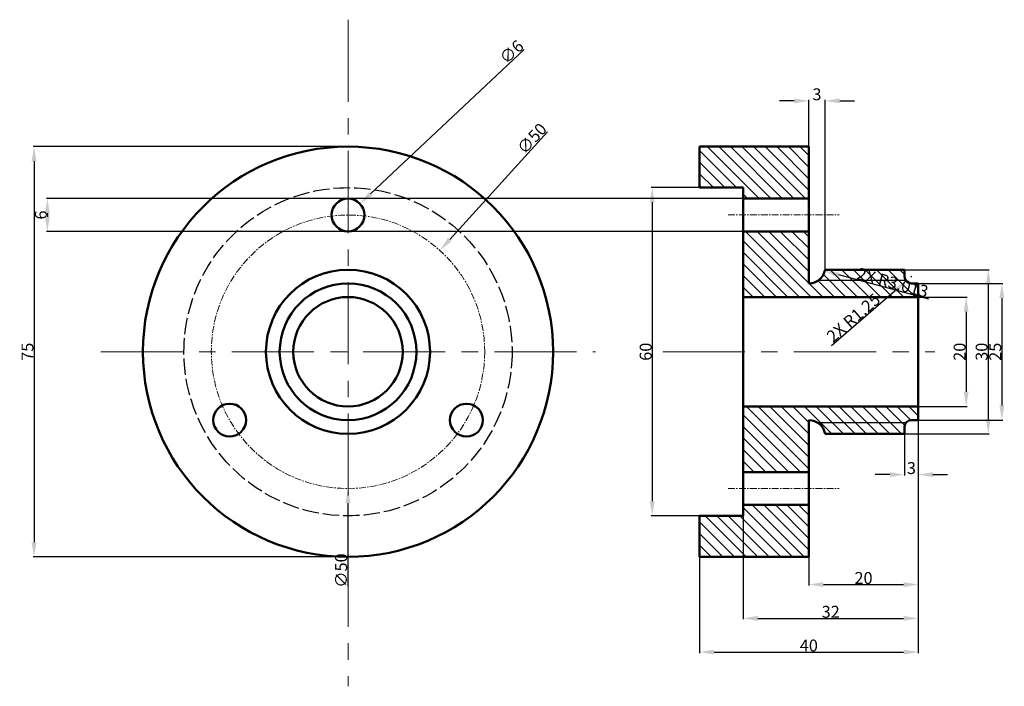
# Model space of a CAD drawing. Units: millimetres. Extents: x 379 to 559, y 190 to 312.
import ezdxf

# ---------------------------------------------------------------- set-up
doc = ezdxf.new("R2010")
doc.units = ezdxf.units.MM
doc.header["$MEASUREMENT"] = 0
doc.linetypes.add('ACAD_ISO02W100', pattern=[15, 12, -3])
doc.linetypes.add('CENTER', pattern=[2, 1.25, -0.25, 0.25, -0.25])
for name, color, linetype, lineweight in [('M-CNTR', 4, 'CENTER', 18), ('M-DIMS', 2, 'Continuous', 25), ('M-HATC', 8, 'Continuous', 18), ('M-HIDN', 3, 'ACAD_ISO02W100', 25), ('M-OUTL', 7, 'Continuous', 50), ('M-THRD', 7, 'Continuous', 25)]:
    doc.layers.add(name, color=color, linetype=linetype, lineweight=lineweight)
doc.styles.get("Standard").update_dxf_attribs({"font": 'arial.ttf'})
doc.dimstyles.get("Standard").update_dxf_attribs({"dimtxt": 2.18, "dimasz": 2.68, "dimexe": 0.18, "dimexo": 0.0625, "dimgap": 0.09, "dimtad": 1, "dimdec": 0, "dimzin": 0, "dimdsep": 46, "dimtxsty": 'Standard', "dimcen": 0.09, "dimadec": 0, "dimazin": 0, "dimtfac": 1, "dimtdec": 0, "dimtofl": 0, "dimtmove": 0, "dimatfit": 3, "dimfxl": 1, "dimtolj": 1, "dimtzin": 0, "dimarcsym": 0})

# ---------------------------------------------------------------- blocks, each defined once
blk = doc.blocks.new('*U1')
blk.add_circle((0, 0), 3)
blk = doc.blocks.new('*U2')
at = {"layer": 'M-OUTL', "color": 0, "linetype": 'ByBlock', "lineweight": -2, "transparency": 16777216}
blk.add_blockref('*U1', (438.8, 276.4), dxfattribs=at)
for p, rotation in [((417.15, 238.9), 120), ((460.45, 238.9), 240)]:
    blk.add_blockref('*U1', p, dxfattribs=dict(at, rotation=rotation))
blk = doc.blocks.new('*D3')
at = {"layer": 'Defpoints', "color": 0, "transparency": 16777216}
for p in [(438.8, 288.9), (381.39, 213.9), (438.8, 213.9)]:
    blk.add_point(p, dxfattribs=at)
at = {"layer": 'M-DIMS', "color": 0, "lineweight": -2, "transparency": 16777216}
for p, q in [((438.74, 288.9), (381.21, 288.9)), ((381.39, 286.22), (381.39, 216.58)), ((438.74, 213.9), (381.21, 213.9))]:
    blk.add_line(p, q, dxfattribs=at)
at = {"layer": 'M-DIMS', "color": 0, "transparency": 16777216}
for points in [[(380.94, 286.22), (381.84, 286.22), (381.39, 288.9)], [(380.94, 216.58), (381.84, 216.58), (381.39, 213.9)]]:
    blk.add_solid(points, dxfattribs=at)
at = {"layer": 'M-DIMS', "color": 0, "transparency": 16777216, "insert": (380.19, 251.4), "char_height": 2.18, "attachment_point": 5, "rotation": 90}
blk.add_mtext('\\A1;75', dxfattribs=at)
blk = doc.blocks.new('*D4')
at = {"layer": 'Defpoints', "color": 0, "transparency": 16777216}
for p in [(440.99, 278.45), (436.61, 274.34)]:
    blk.add_point(p, dxfattribs=at)
at = {"layer": 'M-DIMS', "color": 0, "lineweight": -2, "transparency": 16777216}
for p, q in [((471.01, 306.65), (442.94, 280.29)), ((438.71, 276.4), (438.89, 276.4)), ((438.8, 276.31), (438.8, 276.49))]:
    blk.add_line(p, q, dxfattribs=at)
at = {"layer": 'M-DIMS', "color": 0, "transparency": 16777216}
blk.add_solid([(442.64, 280.61), (443.25, 279.96), (440.99, 278.45)], dxfattribs=at)
at = {"layer": 'M-DIMS', "color": 0, "transparency": 16777216, "insert": (468.7, 306.21), "char_height": 2.18, "attachment_point": 5, "rotation": 43.2019}
blk.add_mtext('\\A1;∅6', dxfattribs=at)
blk = doc.blocks.new('*D5')
at = {"layer": 'Defpoints', "color": 0, "transparency": 16777216}
for p in [(503.07, 281.4), (494.44, 221.4), (503.07, 221.4)]:
    blk.add_point(p, dxfattribs=at)
at = {"layer": 'M-DIMS', "color": 0, "lineweight": -2, "transparency": 16777216}
for p, q in [((503, 281.4), (494.26, 281.4)), ((494.44, 278.72), (494.44, 224.08)), ((503, 221.4), (494.26, 221.4))]:
    blk.add_line(p, q, dxfattribs=at)
at = {"layer": 'M-DIMS', "color": 0, "transparency": 16777216}
for points in [[(493.99, 278.72), (494.88, 278.72), (494.44, 281.4)], [(493.99, 224.08), (494.88, 224.08), (494.44, 221.4)]]:
    blk.add_solid(points, dxfattribs=at)
at = {"layer": 'M-DIMS', "color": 0, "transparency": 16777216, "insert": (493.23, 251.4), "char_height": 2.18, "attachment_point": 5, "rotation": 90}
blk.add_mtext('\\A1;60', dxfattribs=at)
blk = doc.blocks.new('*D6')
at = {"layer": 'Defpoints', "color": 0, "transparency": 16777216}
for p in [(523.07, 297.26), (523.07, 266.4), (526.03, 266.4)]:
    blk.add_point(p, dxfattribs=at)
at = {"layer": 'M-DIMS', "color": 0, "lineweight": -2, "transparency": 16777216}
for p, q in [((520.39, 297.26), (517.71, 297.26)), ((523.07, 266.46), (523.07, 297.44)), ((526.03, 266.46), (526.03, 297.44)), ((528.71, 297.26), (531.39, 297.26))]:
    blk.add_line(p, q, dxfattribs=at)
at = {"layer": 'M-DIMS', "color": 0, "transparency": 16777216}
for points in [[(520.39, 297.71), (520.39, 296.81), (523.07, 297.26)], [(528.71, 297.71), (528.71, 296.81), (526.03, 297.26)]]:
    blk.add_solid(points, dxfattribs=at)
at = {"layer": 'M-DIMS', "color": 0, "transparency": 16777216, "insert": (524.55, 298.46), "char_height": 2.18, "attachment_point": 5}
blk.add_mtext('\\A1;3', dxfattribs=at)
blk = doc.blocks.new('*D7')
at = {"layer": 'Defpoints', "color": 0, "transparency": 16777216}
for p in [(543.07, 261.4), (543.07, 241.4), (551.84, 241.4)]:
    blk.add_point(p, dxfattribs=at)
at = {"layer": 'M-DIMS', "color": 0, "lineweight": -2, "transparency": 16777216}
for p, q in [((543.13, 261.4), (552.02, 261.4)), ((551.84, 258.72), (551.84, 244.08)), ((543.13, 241.4), (552.02, 241.4))]:
    blk.add_line(p, q, dxfattribs=at)
at = {"layer": 'M-DIMS', "color": 0, "transparency": 16777216}
for points in [[(551.39, 258.72), (552.29, 258.72), (551.84, 261.4)], [(551.39, 244.08), (552.29, 244.08), (551.84, 241.4)]]:
    blk.add_solid(points, dxfattribs=at)
at = {"layer": 'M-DIMS', "color": 0, "transparency": 16777216, "insert": (550.64, 251.4), "char_height": 2.18, "attachment_point": 5, "rotation": 90}
blk.add_mtext('\\A1;20', dxfattribs=at)
blk = doc.blocks.new('*D8')
at = {"layer": 'Defpoints', "color": 0, "transparency": 16777216}
for p in [(543.07, 263.9), (543.07, 238.9), (558.37, 238.9)]:
    blk.add_point(p, dxfattribs=at)
at = {"layer": 'M-DIMS', "color": 0, "lineweight": -2, "transparency": 16777216}
for p, q in [((543.13, 263.9), (558.55, 263.9)), ((558.37, 261.22), (558.37, 241.58)), ((543.13, 238.9), (558.55, 238.9))]:
    blk.add_line(p, q, dxfattribs=at)
at = {"layer": 'M-DIMS', "color": 0, "transparency": 16777216}
for points in [[(557.92, 261.22), (558.81, 261.22), (558.37, 263.9)], [(557.92, 241.58), (558.81, 241.58), (558.37, 238.9)]]:
    blk.add_solid(points, dxfattribs=at)
at = {"layer": 'M-DIMS', "color": 0, "transparency": 16777216, "insert": (557.16, 251.4), "char_height": 2.18, "attachment_point": 5, "rotation": 90}
blk.add_mtext('\\A1;25', dxfattribs=at)
blk = doc.blocks.new('*D9')
at = {"layer": 'Defpoints', "color": 0, "transparency": 16777216}
for p in [(543.07, 238.9), (540.57, 236.4), (543.07, 228.93)]:
    blk.add_point(p, dxfattribs=at)
at = {"layer": 'M-DIMS', "color": 0, "lineweight": -2, "transparency": 16777216}
for p, q in [((543.07, 238.84), (543.07, 228.75)), ((540.57, 236.34), (540.57, 228.75)), ((537.89, 228.93), (535.21, 228.93)), ((545.75, 228.93), (548.43, 228.93))]:
    blk.add_line(p, q, dxfattribs=at)
at = {"layer": 'M-DIMS', "color": 0, "transparency": 16777216}
for points in [[(537.89, 229.38), (537.89, 228.48), (540.57, 228.93)], [(545.75, 229.38), (545.75, 228.48), (543.07, 228.93)]]:
    blk.add_solid(points, dxfattribs=at)
at = {"layer": 'M-DIMS', "color": 0, "transparency": 16777216, "insert": (541.82, 230.13), "char_height": 2.18, "attachment_point": 5}
blk.add_mtext('\\A1;3', dxfattribs=at)
blk = doc.blocks.new('*D10')
at = {"layer": 'Defpoints', "color": 0, "transparency": 16777216}
for p in [(543.07, 238.9), (523.07, 213.9), (543.07, 208.84)]:
    blk.add_point(p, dxfattribs=at)
at = {"layer": 'M-DIMS', "color": 0, "lineweight": -2, "transparency": 16777216}
for p, q in [((543.07, 238.84), (543.07, 208.66)), ((523.07, 213.84), (523.07, 208.66)), ((525.75, 208.84), (540.39, 208.84))]:
    blk.add_line(p, q, dxfattribs=at)
at = {"layer": 'M-DIMS', "color": 0, "transparency": 16777216}
for points in [[(525.75, 209.28), (525.75, 208.39), (523.07, 208.84)], [(540.39, 209.28), (540.39, 208.39), (543.07, 208.84)]]:
    blk.add_solid(points, dxfattribs=at)
at = {"layer": 'M-DIMS', "color": 0, "transparency": 16777216, "insert": (533.07, 210.04), "char_height": 2.18, "attachment_point": 5}
blk.add_mtext('\\A1;20', dxfattribs=at)
blk = doc.blocks.new('*D11')
at = {"layer": 'Defpoints', "color": 0, "transparency": 16777216}
for p in [(543.07, 238.9), (511.07, 221.4), (543.07, 202.66)]:
    blk.add_point(p, dxfattribs=at)
at = {"layer": 'M-DIMS', "color": 0, "lineweight": -2, "transparency": 16777216}
for p, q in [((543.07, 238.84), (543.07, 202.48)), ((511.07, 221.34), (511.07, 202.48)), ((513.75, 202.66), (540.39, 202.66))]:
    blk.add_line(p, q, dxfattribs=at)
at = {"layer": 'M-DIMS', "color": 0, "transparency": 16777216}
for points in [[(513.75, 203.1), (513.75, 202.21), (511.07, 202.66)], [(540.39, 203.1), (540.39, 202.21), (543.07, 202.66)]]:
    blk.add_solid(points, dxfattribs=at)
at = {"layer": 'M-DIMS', "color": 0, "transparency": 16777216, "insert": (527.07, 203.86), "char_height": 2.18, "attachment_point": 5}
blk.add_mtext('\\A1;32', dxfattribs=at)
blk = doc.blocks.new('*D12')
at = {"layer": 'Defpoints', "color": 0, "transparency": 16777216}
for p in [(543.07, 238.9), (503.07, 213.9), (543.07, 196.5)]:
    blk.add_point(p, dxfattribs=at)
at = {"layer": 'M-DIMS', "color": 0, "lineweight": -2, "transparency": 16777216}
for p, q in [((543.07, 238.84), (543.07, 196.32)), ((503.07, 213.84), (503.07, 196.32)), ((505.75, 196.5), (540.39, 196.5))]:
    blk.add_line(p, q, dxfattribs=at)
at = {"layer": 'M-DIMS', "color": 0, "transparency": 16777216}
for points in [[(505.75, 196.95), (505.75, 196.05), (503.07, 196.5)], [(540.39, 196.95), (540.39, 196.05), (543.07, 196.5)]]:
    blk.add_solid(points, dxfattribs=at)
at = {"layer": 'M-DIMS', "color": 0, "transparency": 16777216, "insert": (523.07, 197.7), "char_height": 2.18, "attachment_point": 5}
blk.add_mtext('\\A1;40', dxfattribs=at)
blk = doc.blocks.new('*D13')
at = {"layer": 'Defpoints', "color": 0, "transparency": 16777216}
for p in [(455.6, 269.92), (422.01, 232.88)]:
    blk.add_point(p, dxfattribs=at)
at = {"layer": 'M-DIMS', "color": 0, "lineweight": -2, "transparency": 16777216}
for p, q in [((475.27, 291.62), (457.4, 271.9)), ((438.71, 251.4), (438.89, 251.4)), ((438.8, 251.31), (438.8, 251.49))]:
    blk.add_line(p, q, dxfattribs=at)
at = {"layer": 'M-DIMS', "color": 0, "transparency": 16777216}
blk.add_solid([(457.07, 272.2), (457.73, 271.6), (455.6, 269.92)], dxfattribs=at)
at = {"layer": 'M-DIMS', "color": 0, "transparency": 16777216, "insert": (472.43, 290.37), "char_height": 2.18, "attachment_point": 5, "rotation": 47.7955}
blk.add_mtext('\\A1;∅50', dxfattribs=at)
blk = doc.blocks.new('*D14')
at = {"layer": 'Defpoints', "color": 0, "transparency": 16777216}
for p in [(511.07, 279.4), (383.82, 273.4), (511.07, 273.4)]:
    blk.add_point(p, dxfattribs=at)
at = {"layer": 'M-DIMS', "color": 0, "lineweight": -2, "transparency": 16777216}
for p, q in [((511, 279.4), (383.64, 279.4)), ((383.82, 276.72), (383.82, 276.08)), ((511, 273.4), (383.64, 273.4))]:
    blk.add_line(p, q, dxfattribs=at)
at = {"layer": 'M-DIMS', "color": 0, "transparency": 16777216}
for points in [[(383.37, 276.72), (384.27, 276.72), (383.82, 279.4)], [(383.37, 276.08), (384.27, 276.08), (383.82, 273.4)]]:
    blk.add_solid(points, dxfattribs=at)
at = {"layer": 'M-DIMS', "color": 0, "transparency": 16777216, "insert": (382.62, 276.4), "char_height": 2.18, "attachment_point": 5, "rotation": 90}
blk.add_mtext('\\A1;6', dxfattribs=at)
blk = doc.blocks.new('*D15')
at = {"layer": 'Defpoints', "color": 0, "transparency": 16777216}
for p in [(540.57, 266.4), (540.57, 236.4), (555.88, 236.4)]:
    blk.add_point(p, dxfattribs=at)
at = {"layer": 'M-DIMS', "color": 0, "lineweight": -2, "transparency": 16777216}
for p, q in [((540.63, 266.4), (556.06, 266.4)), ((555.88, 263.72), (555.88, 239.08)), ((540.63, 236.4), (556.06, 236.4))]:
    blk.add_line(p, q, dxfattribs=at)
at = {"layer": 'M-DIMS', "color": 0, "transparency": 16777216}
for points in [[(555.43, 263.72), (556.33, 263.72), (555.88, 266.4)], [(555.43, 239.08), (556.33, 239.08), (555.88, 236.4)]]:
    blk.add_solid(points, dxfattribs=at)
at = {"layer": 'M-DIMS', "color": 0, "transparency": 16777216, "insert": (554.67, 251.4), "char_height": 2.18, "attachment_point": 5, "rotation": 90}
blk.add_mtext('\\A1;30', dxfattribs=at)
blk = doc.blocks.new('*D16')
at = {"layer": 'Defpoints', "color": 0, "transparency": 16777216}
for p in [(438.8, 276.4), (438.8, 226.4)]:
    blk.add_point(p, dxfattribs=at)
at = {"layer": 'M-DIMS', "color": 0, "lineweight": -2, "transparency": 16777216}
for p, q in [((438.71, 251.4), (438.89, 251.4)), ((438.8, 251.31), (438.8, 251.49)), ((438.8, 208.56), (438.8, 223.72))]:
    blk.add_line(p, q, dxfattribs=at)
at = {"layer": 'M-DIMS', "color": 0, "transparency": 16777216}
blk.add_solid([(438.35, 223.72), (439.25, 223.72), (438.8, 226.4)], dxfattribs=at)
at = {"layer": 'M-DIMS', "color": 0, "transparency": 16777216, "insert": (437.54, 211.4), "char_height": 2.18, "attachment_point": 5, "rotation": 89.997}
blk.add_mtext('\\A1;∅50', dxfattribs=at)
blk = doc.blocks.new('*D17')
at = {"layer": 'Defpoints', "color": 0, "transparency": 16777216}
for p in [(523.07, 266.91), (525.97, 266.13)]:
    blk.add_point(p, dxfattribs=at)
at = {"layer": 'M-DIMS', "color": 0, "lineweight": -2, "transparency": 16777216}
for p, q in [((522.98, 266.91), (523.16, 266.91)), ((523.07, 266.82), (523.07, 267)), ((545, 261.01), (528.56, 265.43))]:
    blk.add_line(p, q, dxfattribs=at)
at = {"layer": 'M-DIMS', "color": 0, "transparency": 16777216}
blk.add_solid([(528.68, 265.86), (528.45, 265), (525.97, 266.13)], dxfattribs=at)
at = {"layer": 'M-DIMS', "color": 0, "transparency": 16777216, "insert": (538.39, 264.04), "char_height": 2.18, "attachment_point": 5, "rotation": 344.9428}
blk.add_mtext('\\A1;2X R3.013', dxfattribs=at)
blk = doc.blocks.new('*D18')
at = {"layer": 'Defpoints', "color": 0, "transparency": 16777216}
for p in [(541.82, 265.15), (540.87, 264.33)]:
    blk.add_point(p, dxfattribs=at)
at = {"layer": 'M-DIMS', "color": 0, "lineweight": -2, "transparency": 16777216}
for p, q in [((541.73, 265.15), (541.91, 265.15)), ((541.82, 265.06), (541.82, 265.24)), ((527.21, 252.57), (538.84, 262.58))]:
    blk.add_line(p, q, dxfattribs=at)
at = {"layer": 'M-DIMS', "color": 0, "transparency": 16777216}
blk.add_solid([(538.55, 262.92), (539.13, 262.24), (540.87, 264.33)], dxfattribs=at)
at = {"layer": 'M-DIMS', "color": 0, "transparency": 16777216, "insert": (531.22, 257.61), "char_height": 2.18, "attachment_point": 5, "rotation": 40.7501}
blk.add_mtext('\\A1;2X R1.25', dxfattribs=at)

msp = doc.modelspace()

# ---------------------------------------------------------------- hatches: boundary and pattern name
at = {"layer": 'M-HATC'}
h = msp.add_hatch(dxfattribs=at)
h.set_pattern_fill('ANSI31', color=256, scale=12, angle=90)
h.paths.add_polyline_path([(523.0651, 288.8985), (503.0651, 288.8985), (503.0651, 281.3985), (511.0651, 281.3985), (511.0651, 279.3985), (523.0651, 279.3985)])
h = msp.add_hatch(dxfattribs=at)
h.set_pattern_fill('ANSI31', color=256, scale=12, angle=90)
h.paths.add_polyline_path([(523.0651, 273.3985), (511.0651, 273.3985), (511.0651, 261.3985), (543.0651, 261.3985), (543.0651, 263.8985), (541.8151, 263.8985, -0.23606798), (540.8151, 264.3985), (524.7273, 264.3985, -0.14714445), (523.0651, 263.8985)])
h.paths.add_polyline_path([(523.0651, 238.8985, -0.14714445), (524.7273, 238.3985), (540.8151, 238.3985, -0.23606798), (541.8151, 238.8985), (543.0651, 238.8985), (543.0651, 241.3985), (511.0651, 241.3985), (511.0651, 229.3985), (523.0651, 229.3985)])
h.paths.add_polyline_path([(523.0651, 223.3985), (511.0651, 223.3985), (511.0651, 221.3985), (503.0651, 221.3985), (503.0651, 213.8985), (523.0651, 213.8985)])
h.paths.add_polyline_path([(540.5651, 237.6485, -0.16227766), (540.8151, 238.3985), (524.7273, 238.3985, -0.20670025), (526.0341, 236.3985), (540.5651, 236.3985)], flags=17)
h.paths.add_polyline_path([(540.5651, 266.3985), (526.0341, 266.3985, -0.20670025), (524.7273, 264.3985), (540.8151, 264.3985, -0.16227766), (540.5651, 265.1485)], flags=17)

# ---------------------------------------------------------------- linework, layer by layer
at = {"layer": 'M-CNTR', "ltscale": 12}
for p, q in [((438.8013, 312.1028), (438.8013, 190.2367)), ((393.5709, 251.3985), (484.0317, 251.3985)), ((496.3528, 251.3985), (546.1285, 251.3985))]:
    msp.add_line(p, q, dxfattribs=at)
at = {"layer": 'M-CNTR'}
for p, q in [((508.2988, 276.3985), (528.6442, 276.3985)), ((508.2988, 226.3985), (528.6442, 226.3985))]:
    msp.add_line(p, q, dxfattribs=at)
msp.add_circle((438.8013, 251.3985), 25, dxfattribs=at)
msp.add_circle((438.8013, 251.3985), 25, dxfattribs=at)
at = {"layer": 'M-HIDN', "ltscale": 0.25}
msp.add_circle((438.8013, 251.3985), 30, dxfattribs=at)
at = {"layer": 'M-OUTL'}
for p, q in [((503.0651, 281.3985), (503.0651, 288.8985)), ((503.0651, 288.8985), (523.0651, 288.8985)), ((523.0651, 288.8985), (523.0651, 263.8985)), ((511.0651, 281.3985), (503.0651, 281.3985)), ((511.0651, 281.3985), (511.0651, 221.3985)), ((511.0651, 221.3985), (511.0651, 281.3985)), ((511.0651, 279.3985), (523.0651, 279.3985)), ((511.0651, 273.3985), (523.0651, 273.3985)), ((540.5651, 266.3985), (526.0341, 266.3985)), ((540.5651, 265.1485), (540.5651, 266.3985)), ((511.0651, 251.3985), (511.0651, 263.8985)), ((541.8151, 263.8985), (543.0651, 263.8985)), ((543.0651, 263.8985), (541.8151, 263.8985)), ((543.0651, 238.8985), (543.0651, 263.8985)), ((543.0651, 251.3985), (543.0651, 263.8985)), ((511.0651, 251.3985), (511.0651, 261.3985)), ((511.0651, 261.3985), (543.0651, 261.3985)), ((526.0651, 261.3985), (543.0651, 261.3985)), ((511.0651, 251.3985), (511.0651, 241.3985)), ((511.0651, 251.3985), (511.0651, 238.8985)), ((511.0651, 241.3985), (543.0651, 241.3985)), ((511.0651, 241.3985), (543.0651, 241.3985)), ((526.0651, 241.3985), (543.0651, 241.3985)), ((523.0651, 213.8985), (523.0651, 238.8985)), ((523.0651, 213.8985), (523.0651, 238.8985)), ((541.8151, 238.8985), (543.0651, 238.8985)), ((543.0651, 238.8985), (541.8151, 238.8985)), ((540.5651, 236.3985), (526.0341, 236.3985)), ((540.5651, 237.6485), (540.5651, 236.3985)), ((511.0651, 229.3985), (523.0651, 229.3985)), ((511.0651, 223.3985), (523.0651, 223.3985)), ((511.0651, 221.3985), (503.0651, 221.3985)), ((503.0651, 221.3985), (503.0651, 213.8985)), ((511.0651, 221.3985), (503.0651, 221.3985)), ((503.0651, 221.3985), (503.0651, 213.8985)), ((503.0651, 213.8985), (523.0651, 213.8985)), ((503.0651, 213.8985), (523.0651, 213.8985))]:
    msp.add_line(p, q, dxfattribs=at)
for radius in [37.5, 15, 12.5, 10]:
    msp.add_circle((438.8013, 251.3985), radius, dxfattribs=at)
for centre, radius, start, end in [((523.0651, 266.9115), 3.013, 270, 350.197086), ((541.8151, 265.1485), 1.25, 180, 270), ((523.0651, 235.8855), 3.013, 9.802914, 90), ((541.8151, 237.6485), 1.25, 90, 180)]:
    msp.add_arc(centre, radius, start, end, dxfattribs=at)
at = {"layer": 'M-THRD'}
for p, q in [((540.8151, 264.3985), (524.7273, 264.3985)), ((540.8151, 238.3985), (524.7273, 238.3985))]:
    msp.add_line(p, q, dxfattribs=at)

# ---------------------------------------------------------------- block references
at = {"layer": 'M-OUTL'}
msp.add_blockref('*U2', (0, 0), dxfattribs=at)

# ---------------------------------------------------------------- dimensions: what is measured, and where the dimension line sits
at = {"layer": 'M-DIMS'}
for p1, p2, override, picture, middle in [((436.6145, 274.3448), (440.9882, 278.4522), {"dimclrd": 0, "dimclre": 0, "dimclrt": 0}, '*D4', (469.5614, 305.286)), ((422.0069, 232.8797), (455.5958, 269.9173), {"dimclrd": 0, "dimclre": 0, "dimclrt": 0}, '*D13', (473.37, 289.5165)), ((438.8026, 276.3985), (438.8, 226.3985), {"dimdec": 0, "dimlfac": 1, "dimrnd": 0, "dimzin": 0, "dimdsep": 46, "dimlunit": 2}, '*D16', (438.7992, 211.3985))]:
    dim = msp.add_diameter_dim_2p(p1=p1, p2=p2, dimstyle='Standard', override=override, dxfattribs=at)
    dim.commit()
    dim.dimension.update_dxf_attribs({"geometry": picture, "text_midpoint": middle, "dimtype": 163})
for base, p1, p2, picture, middle in [((523.0651, 297.2591), (526.0341, 266.3985), (523.0651, 266.3985), '*D6', (524.5496, 298.4629)), ((543.0651, 196.4993), (503.0651, 213.8985), (543.0651, 238.8985), '*D12', (523.0651, 197.7023)), ((543.0651, 202.6556), (511.0651, 221.3985), (543.0651, 238.8985), '*D11', (527.0651, 203.8594)), ((543.0651, 208.8353), (523.0651, 213.8985), (543.0651, 238.8985), '*D10', (533.0651, 210.0384)), ((543.0650851235, 228.9309314688), (540.5650851235, 236.3984917377), (543.0650851235, 238.8984917377), '*D9', (541.8150851235, 230.1347241019))]:
    dim = msp.add_linear_dim(base=base, p1=p1, p2=p2, dimstyle='Standard', override={"dimclrd": 0, "dimclre": 0, "dimclrt": 0}, dxfattribs=at)
    dim.commit()
    dim.dimension.update_dxf_attribs({"geometry": picture, "text_midpoint": middle})
for base, p1, p2, override, picture, middle in [((381.3912, 213.8985), (438.8013, 288.8985), (438.8013, 213.8985), {"dimclrd": 0, "dimclre": 0, "dimclrt": 0}, '*D3', (380.1926, 251.3985)), ((494.4372, 221.3985), (503.0651, 281.3985), (503.0651, 221.3985), {"dimclrd": 0, "dimclre": 0, "dimclrt": 0}, '*D5', (493.2342, 251.3985)), ((383.8209, 273.3985), (511.0651, 279.3985), (511.0651, 273.3985), {"dimdec": 0, "dimlfac": 1, "dimrnd": 0, "dimzin": 0, "dimdsep": 46, "dimlunit": 2}, '*D14', (382.6179, 276.3985)), ((555.8785, 236.3985), (540.5651, 266.3985), (540.5651, 236.3985), {"dimdec": 0, "dimlfac": 1, "dimrnd": 0, "dimzin": 0, "dimdsep": 46, "dimlunit": 2}, '*D15', (554.6747, 251.3985)), ((558.3672, 238.8985), (543.0651, 263.8985), (543.0651, 238.8985), {"dimclrd": 0, "dimclre": 0, "dimclrt": 0}, '*D8', (557.1642, 251.3985)), ((551.8389, 241.3985), (543.0651, 261.3985), (543.0651, 241.3985), {"dimclrd": 0, "dimclre": 0, "dimclrt": 0}, '*D7', (550.6359, 251.3985))]:
    dim = msp.add_linear_dim(base=base, p1=p1, p2=p2, angle=90, dimstyle='Standard', override=override, dxfattribs=at)
    dim.commit()
    dim.dimension.update_dxf_attribs({"geometry": picture, "text_midpoint": middle})
for center, mpoint, override, picture, middle in [((523.0651, 266.9115), (525.9746, 266.1288), {"dimdec": 3, "dimlfac": 1, "dimrnd": 0, "dimzin": 0, "dimdsep": 46, "dimlunit": 2}, '*D17', (538.3891, 264.0356)), ((541.8151, 265.1485), (540.8681, 264.3325), {"dimdec": 2, "dimlfac": 1, "dimrnd": 0, "dimzin": 0, "dimdsep": 46, "dimlunit": 2}, '*D18', (531.2244, 257.611))]:
    dim = msp.add_radius_dim(center=center, mpoint=mpoint, text='2X <>', dimstyle='Standard', override=override, dxfattribs=at)
    dim.commit()
    dim.dimension.update_dxf_attribs({"geometry": picture, "text_midpoint": middle})

doc.saveas('drawing.dxf')
